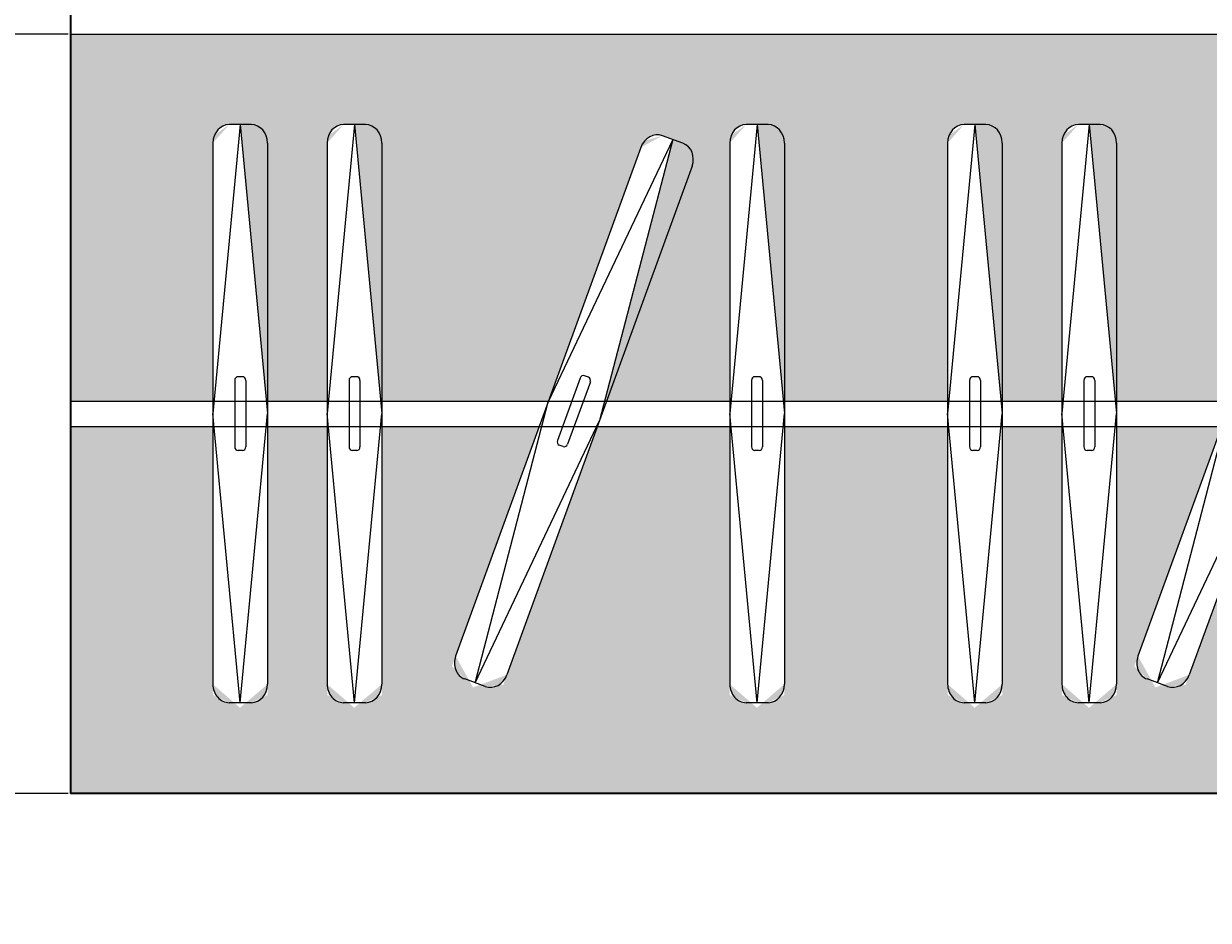
# Model space of a CAD drawing. Units: millimetres. Extents: x 27017497 to 27018854, y 7058029 to 7059154.
# Tile 38 of 91: x 27017621 to 27017655, y 7058433 to 7058459. Entities that reach past the tile are written whole.
import ezdxf

# ---------------------------------------------------------------- set-up
doc = ezdxf.new("R2010")
doc.units = ezdxf.units.MM
for name, color, linetype, lineweight in [('A-ANNO-DIMS', 2, 'Continuous', 18), ('A-FLOR-CASE', 8, 'Continuous', 20), ('A-FLOR-CASE-PATT', 44, 'Continuous', 13), ('A-WALL', 7, 'Continuous', 35)]:
    doc.layers.add(name, color=color, linetype=linetype, lineweight=lineweight)
doc.styles.get("Standard").update_dxf_attribs({"font": 'arial.ttf'})
doc.dimstyles.get("Standard").update_dxf_attribs({"dimtxt": 0.18, "dimasz": 0.18, "dimexe": 0.18, "dimexo": 0.0625, "dimgap": 0.09, "dimtad": 0, "dimtih": 1, "dimtoh": 1, "dimdec": 4, "dimzin": 0, "dimdsep": 46, "dimtxsty": 'Standard', "dimcen": 0.09, "dimadec": 0, "dimazin": 0, "dimtfac": 1, "dimtdec": 4, "dimtofl": 0, "dimtmove": 0, "dimatfit": 3, "dimfxl": 1, "dimtolj": 1, "dimtzin": 0, "dimarcsym": 0})

# ---------------------------------------------------------------- blocks, each defined once
blk = doc.blocks.new('WARDROBE-HANGING-WALL-BACKED')
for p, q in [((0, 21.737), (65.212, 21.737)), ((0, 0), (0, 21.737)), ((4.862, 19.152), (4.08, 10.877)), ((5.175, 19.152), (4.549, 19.152)), ((4.862, 19.152), (5.645, 10.877)), ((8.135, 19.152), (7.353, 10.877)), ((8.448, 19.152), (7.822, 19.152)), ((8.135, 19.152), (8.918, 10.877)), ((19.663, 19.152), (18.88, 10.877)), ((19.976, 19.152), (19.35, 19.152)), ((19.663, 19.152), (20.445, 10.877)), ((25.9, 19.152), (25.118, 10.877)), ((26.213, 19.152), (25.587, 19.152)), ((25.9, 19.152), (26.683, 10.877)), ((29.173, 19.152), (28.391, 10.877)), ((29.486, 19.152), (28.86, 19.152)), ((29.173, 19.152), (29.956, 10.877)), ((17.246, 18.725), (13.68, 11.217)), ((17.246, 18.725), (15.151, 10.682)), ((17.54, 18.618), (16.952, 18.833)), ((4.08, 18.624), (4.08, 3.13)), ((5.645, 18.624), (5.645, 3.13)), ((7.353, 18.624), (7.353, 3.13)), ((8.918, 18.624), (8.918, 3.13)), ((16.33, 18.497), (11.03, 3.937)), ((18.88, 18.624), (18.88, 3.13)), ((20.445, 18.624), (20.445, 3.13)), ((25.118, 18.624), (25.118, 3.13)), ((26.683, 18.624), (26.683, 3.13)), ((28.391, 18.624), (28.391, 3.13)), ((29.956, 18.624), (29.956, 3.13)), ((35.867, 18.497), (30.567, 3.937)), ((17.8, 17.961), (12.501, 3.402)), ((37.337, 17.961), (32.038, 3.402)), ((4.925, 11.933), (4.8, 11.933)), ((8.198, 11.933), (8.073, 11.933)), ((14.594, 11.896), (13.943, 10.109)), ((14.836, 11.92), (14.718, 11.963)), ((19.725, 11.933), (19.6, 11.933)), ((25.963, 11.933), (25.838, 11.933)), ((29.236, 11.933), (29.111, 11.933)), ((4.706, 11.828), (4.706, 9.926)), ((5.019, 11.828), (5.019, 9.926)), ((7.979, 11.828), (7.979, 9.926)), ((8.292, 11.828), (8.292, 9.926)), ((14.888, 11.789), (14.237, 10.002)), ((19.506, 11.828), (19.506, 9.926)), ((19.819, 11.828), (19.819, 9.926)), ((25.744, 11.828), (25.744, 9.926)), ((26.057, 11.828), (26.057, 9.926)), ((29.017, 11.828), (29.017, 9.926)), ((29.33, 11.828), (29.33, 9.926)), ((0, 11.231), (65.212, 11.231)), ((11.585, 3.173), (13.68, 11.217)), ((31.122, 3.173), (33.217, 11.217)), ((4.862, 2.602), (4.08, 10.877)), ((4.862, 2.602), (5.645, 10.877)), ((8.135, 2.602), (7.353, 10.877)), ((8.135, 2.602), (8.918, 10.877)), ((19.663, 2.602), (18.88, 10.877)), ((19.663, 2.602), (20.445, 10.877)), ((25.9, 2.602), (25.118, 10.877)), ((25.9, 2.602), (26.683, 10.877)), ((29.173, 2.602), (28.391, 10.877)), ((29.173, 2.602), (29.956, 10.877)), ((11.585, 3.173), (15.151, 10.682)), ((31.122, 3.173), (34.688, 10.682)), ((0, 10.506), (65.212, 10.506)), ((14.113, 9.935), (13.995, 9.978)), ((4.925, 9.821), (4.8, 9.821)), ((8.198, 9.821), (8.073, 9.821)), ((19.725, 9.821), (19.6, 9.821)), ((25.963, 9.821), (25.838, 9.821)), ((29.236, 9.821), (29.111, 9.821)), ((11.879, 3.066), (11.291, 3.28)), ((31.416, 3.066), (30.828, 3.28)), ((5.175, 2.602), (4.549, 2.602)), ((8.448, 2.602), (7.822, 2.602)), ((19.976, 2.602), (19.35, 2.602)), ((26.213, 2.602), (25.587, 2.602)), ((29.486, 2.602), (28.86, 2.602))]:
    blk.add_line(p, q)
for centre, major_axis, start_param, end_param in [((4.549, 18.624), (0, 0.528), 0, 1.570796), ((5.175, 18.624), (0, 0.528), 4.712389, 6.283185), ((7.822, 18.624), (0, 0.528), 0, 1.570796), ((8.448, 18.624), (0, 0.528), 4.712389, 6.283185), ((19.35, 18.624), (0, 0.528), 0, 1.570796), ((19.976, 18.624), (0, 0.528), 4.712389, 6.283185), ((25.587, 18.624), (0, 0.528), 0, 1.570796), ((26.213, 18.624), (0, 0.528), 4.712389, 6.283185), ((28.86, 18.624), (0, 0.528), 0, 1.570796), ((29.486, 18.624), (0, 0.528), 4.712389, 6.283185), ((16.771, 18.336), (0.181, 0.496), 0, 1.570796), ((17.359, 18.122), (0.181, 0.496), -1.570796, 0), ((4.8, 11.828), (0, 0.106), 0, 1.570796), ((4.925, 11.828), (0, 0.106), -1.570796, 0), ((8.073, 11.828), (0, 0.106), 0, 1.570796), ((8.198, 11.828), (0, 0.106), -1.570796, 0), ((14.682, 11.864), (0.0361, 0.0993), 0, 1.570796), ((14.799, 11.821), (0.0361, 0.0993), 4.712389, 6.283185), ((19.6, 11.828), (0, 0.106), 0, 1.570796), ((19.725, 11.828), (0, 0.106), -1.570796, 0), ((25.838, 11.828), (0, 0.106), 0, 1.570796), ((25.963, 11.828), (0, 0.106), -1.570796, 0), ((29.111, 11.828), (0, 0.106), 0, 1.570796), ((29.236, 11.828), (0, 0.106), -1.570796, 0), ((4.8, 9.926), (0, 0.106), 1.570796, 3.141593), ((4.925, 9.926), (0, 0.106), 3.141593, 4.712389), ((8.073, 9.926), (0, 0.106), 1.570796, 3.141593), ((8.198, 9.926), (0, 0.106), 3.141593, 4.712389), ((14.031, 10.077), (0.0361, 0.0993), 1.570796, 3.141593), ((14.149, 10.034), (0.0361, 0.0993), 3.141593, 4.712389), ((19.6, 9.926), (0, 0.106), 1.570796, 3.141593), ((19.725, 9.926), (0, 0.106), 3.141593, 4.712389), ((25.838, 9.926), (0, 0.106), 1.570796, 3.141593), ((25.963, 9.926), (0, 0.106), 3.141593, 4.712389), ((29.111, 9.926), (0, 0.106), 1.570796, 3.141593), ((29.236, 9.926), (0, 0.106), 3.141593, 4.712389), ((11.472, 3.776), (0.181, 0.496), 1.570796, 3.141593), ((31.008, 3.776), (0.181, 0.496), 1.570796, 3.141593), ((12.06, 3.562), (0.181, 0.496), 3.141593, 4.712389), ((31.597, 3.562), (0.181, 0.496), 3.141593, 4.712389), ((4.549, 3.13), (0, 0.528), 1.570796, 3.141593), ((5.175, 3.13), (0, 0.528), 3.141593, 4.712389), ((7.822, 3.13), (0, 0.528), 1.570796, 3.141593), ((8.448, 3.13), (0, 0.528), 3.141593, 4.712389), ((19.35, 3.13), (0, 0.528), 1.570796, 3.141593), ((19.976, 3.13), (0, 0.528), 3.141593, 4.712389), ((25.587, 3.13), (0, 0.528), 1.570796, 3.141593), ((26.213, 3.13), (0, 0.528), 3.141593, 4.712389), ((28.86, 3.13), (0, 0.528), 1.570796, 3.141593), ((29.486, 3.13), (0, 0.528), 3.141593, 4.712389)]:
    blk.add_ellipse(centre, major_axis=major_axis, ratio=0.888892, start_param=start_param, end_param=end_param)
blk = doc.blocks.new('*D45')
at = {"layer": 'A-ANNO-DIMS', "color": 0, "lineweight": -2, "transparency": 16777216}
for p, q in [((27017622.665, 7058458.704), (27017622.665, 7058468.604)), ((27017687.877, 7058458.704), (27017687.877, 7058468.604)), ((27017622.845, 7058468.424), (27017653.586, 7058468.424)), ((27017687.697, 7058468.424), (27017656.955, 7058468.424))]:
    blk.add_line(p, q, dxfattribs=at)
at = {"layer": 'A-ANNO-DIMS', "color": 0, "transparency": 16777216}
for points in [[(27017622.845, 7058468.454), (27017622.845, 7058468.394), (27017622.665, 7058468.424)], [(27017687.697, 7058468.454), (27017687.697, 7058468.394), (27017687.877, 7058468.424)]]:
    blk.add_solid(points, dxfattribs=at)
at = {"layer": 'Defpoints', "color": 0, "transparency": 16777216}
for p in [(27017687.877, 7058468.424), (27017622.665, 7058458.642), (27017687.877, 7058458.642)]:
    blk.add_point(p, dxfattribs=at)
at = {"layer": 'A-ANNO-DIMS', "color": 0, "transparency": 16777216, "insert": (27017655.271, 7058468.424), "char_height": 0.18, "attachment_point": 5}
blk.add_mtext('\\A1;WALL WARDROBE 65 TYP.', dxfattribs=at)
blk = doc.blocks.new('*D46')
at = {"layer": 'A-ANNO-DIMS', "color": 0, "lineweight": -2, "transparency": 16777216}
for p, q in [((27017622.603, 7058458.642), (27017612.703, 7058458.642)), ((27017612.883, 7058458.462), (27017612.883, 7058447.954)), ((27017612.883, 7058437.085), (27017612.883, 7058447.593)), ((27017622.603, 7058436.905), (27017612.703, 7058436.905))]:
    blk.add_line(p, q, dxfattribs=at)
at = {"layer": 'A-ANNO-DIMS', "color": 0, "transparency": 16777216}
for points in [[(27017612.853, 7058458.462), (27017612.913, 7058458.462), (27017612.883, 7058458.642)], [(27017612.853, 7058437.085), (27017612.913, 7058437.085), (27017612.883, 7058436.905)]]:
    blk.add_solid(points, dxfattribs=at)
at = {"layer": 'Defpoints', "color": 0, "transparency": 16777216}
for p in [(27017612.883, 7058458.642), (27017622.665, 7058458.642), (27017622.665, 7058436.905)]:
    blk.add_point(p, dxfattribs=at)
at = {"layer": 'A-ANNO-DIMS', "color": 0, "transparency": 16777216, "insert": (27017612.883, 7058447.773), "char_height": 0.18, "attachment_point": 5}
blk.add_mtext('\\A1;22 TYP.', dxfattribs=at)
blk = doc.blocks.new('*D48')
at = {"layer": 'A-ANNO-DIMS', "color": 0, "lineweight": -2, "transparency": 16777216}
for p, q in [((27018463.498, 7058622.912), (27017497.536, 7058622.912)), ((27017497.716, 7058622.732), (27017497.716, 7058357.753)), ((27017497.716, 7058092.41), (27017497.716, 7058357.389)), ((27018555.129, 7058092.23), (27017497.536, 7058092.23))]:
    blk.add_line(p, q, dxfattribs=at)
at = {"layer": 'A-ANNO-DIMS', "color": 0, "transparency": 16777216}
for points in [[(27017497.686, 7058622.732), (27017497.746, 7058622.732), (27017497.716, 7058622.912)], [(27017497.686, 7058092.41), (27017497.746, 7058092.41), (27017497.716, 7058092.23)]]:
    blk.add_solid(points, dxfattribs=at)
at = {"layer": 'Defpoints', "color": 0, "transparency": 16777216}
for p in [(27018463.561, 7058622.912), (27017497.716, 7058092.23), (27018555.192, 7058092.23)]:
    blk.add_point(p, dxfattribs=at)
at = {"layer": 'A-ANNO-DIMS', "color": 0, "transparency": 16777216, "insert": (27017497.716, 7058357.571), "char_height": 0.18, "attachment_point": 5}
blk.add_mtext('\\A1;530.7', dxfattribs=at)

msp = doc.modelspace()

# ---------------------------------------------------------------- hatches: boundary and pattern name
at = {"layer": 'A-FLOR-CASE-PATT'}
h = msp.add_hatch(color=256, dxfattribs=at)
h.dxf.hatch_style = 1
edge = h.paths.add_edge_path()
edge.add_line((27017641.545, 7058447.411), (27017637.752, 7058447.411))
edge.add_line((27017637.752, 7058447.411), (27017635.06, 7058440.016))
edge.add_ellipse((27017634.725, 7058440.467), major_axis=(0.181, 0.496), ratio=0.888892, start_angle=180, end_angle=270, ccw=False)
edge.add_line((27017634.184, 7058439.939), (27017634.19, 7058439.951))
edge.add_ellipse((27017634.137, 7058440.681), major_axis=(0.181, 0.496), ratio=0.888892, start_angle=90, end_angle=180, ccw=False)
edge.add_line((27017633.59, 7058440.551), (27017636.086, 7058447.411))
edge.add_line((27017636.086, 7058447.411), (27017631.583, 7058447.411))
edge.add_line((27017631.583, 7058447.411), (27017631.583, 7058439.726))
edge.add_ellipse((27017631.113, 7058440.035), major_axis=(0, 0.528), ratio=0.888892, start_angle=180, end_angle=270, ccw=False)
edge.add_line((27017630.786, 7058439.354), (27017630.787, 7058439.367))
edge.add_ellipse((27017630.487, 7058440.035), major_axis=(0, 0.528), ratio=0.888892, start_angle=90, end_angle=180, ccw=False)
edge.add_line((27017630.018, 7058439.726), (27017630.018, 7058447.411))
edge.add_line((27017630.018, 7058447.411), (27017628.31, 7058447.411))
edge.add_line((27017628.31, 7058447.411), (27017628.31, 7058439.726))
edge.add_ellipse((27017627.84, 7058440.035), major_axis=(0, 0.528), ratio=0.888892, start_angle=180, end_angle=270, ccw=False)
edge.add_line((27017627.513, 7058439.354), (27017627.514, 7058439.367))
edge.add_ellipse((27017627.214, 7058440.035), major_axis=(0, 0.528), ratio=0.888892, start_angle=90, end_angle=180, ccw=False)
edge.add_line((27017626.745, 7058439.726), (27017626.745, 7058447.411))
edge.add_line((27017626.745, 7058447.411), (27017622.666, 7058447.411))
edge.add_line((27017622.666, 7058447.411), (27017622.666, 7058436.912))
edge.add_line((27017622.666, 7058436.912), (27017687.877, 7058436.912))
edge.add_line((27017687.877, 7058436.912), (27017687.877, 7058447.411))
edge.add_line((27017687.877, 7058447.411), (27017685.741, 7058447.411))
edge.add_line((27017685.741, 7058447.411), (27017685.741, 7058439.726))
edge.add_ellipse((27017685.271, 7058440.035), major_axis=(0, 0.528), ratio=0.888892, start_angle=180, end_angle=270, ccw=False)
edge.add_line((27017684.944, 7058439.354), (27017684.945, 7058439.367))
edge.add_ellipse((27017684.645, 7058440.035), major_axis=(0, 0.528), ratio=0.888892, start_angle=90, end_angle=180, ccw=False)
edge.add_line((27017684.176, 7058439.726), (27017684.176, 7058447.411))
edge.add_line((27017684.176, 7058447.411), (27017680.383, 7058447.411))
edge.add_line((27017680.383, 7058447.411), (27017677.691, 7058440.016))
edge.add_ellipse((27017677.356, 7058440.467), major_axis=(0.181, 0.496), ratio=0.888892, start_angle=180, end_angle=270, ccw=False)
edge.add_line((27017676.815, 7058439.939), (27017676.821, 7058439.951))
edge.add_ellipse((27017676.767, 7058440.681), major_axis=(0.181, 0.496), ratio=0.888892, start_angle=90, end_angle=180, ccw=False)
edge.add_line((27017676.22, 7058440.551), (27017678.717, 7058447.411))
edge.add_line((27017678.717, 7058447.411), (27017674.214, 7058447.411))
edge.add_line((27017674.214, 7058447.411), (27017674.214, 7058439.726))
edge.add_ellipse((27017673.744, 7058440.035), major_axis=(0, 0.528), ratio=0.888892, start_angle=180, end_angle=270, ccw=False)
edge.add_line((27017673.417, 7058439.354), (27017673.418, 7058439.367))
edge.add_ellipse((27017673.118, 7058440.035), major_axis=(0, 0.528), ratio=0.888892, start_angle=90, end_angle=180, ccw=False)
edge.add_line((27017672.649, 7058439.726), (27017672.649, 7058447.411))
edge.add_line((27017672.649, 7058447.411), (27017670.94, 7058447.411))
edge.add_line((27017670.94, 7058447.411), (27017670.94, 7058439.726))
edge.add_ellipse((27017670.471, 7058440.035), major_axis=(0, 0.528), ratio=0.888892, start_angle=180, end_angle=270, ccw=False)
edge.add_line((27017670.143, 7058439.354), (27017670.145, 7058439.367))
edge.add_ellipse((27017669.845, 7058440.035), major_axis=(0, 0.528), ratio=0.888892, start_angle=90, end_angle=180, ccw=False)
edge.add_line((27017669.375, 7058439.726), (27017669.375, 7058447.411))
edge.add_line((27017669.375, 7058447.411), (27017663.036, 7058447.411))
edge.add_line((27017663.036, 7058447.411), (27017663.036, 7058439.726))
edge.add_ellipse((27017662.567, 7058440.035), major_axis=(0, 0.528), ratio=0.888892, start_angle=180, end_angle=270, ccw=False)
edge.add_line((27017662.239, 7058439.354), (27017662.241, 7058439.367))
edge.add_ellipse((27017661.941, 7058440.035), major_axis=(0, 0.528), ratio=0.888892, start_angle=90, end_angle=180, ccw=False)
edge.add_line((27017661.471, 7058439.726), (27017661.471, 7058447.411))
edge.add_line((27017661.471, 7058447.411), (27017657.289, 7058447.411))
edge.add_line((27017657.289, 7058447.411), (27017654.597, 7058440.016))
edge.add_ellipse((27017654.262, 7058440.467), major_axis=(0.181, 0.496), ratio=0.888892, start_angle=180, end_angle=270, ccw=False)
edge.add_line((27017653.721, 7058439.939), (27017653.727, 7058439.951))
edge.add_ellipse((27017653.673, 7058440.681), major_axis=(0.181, 0.496), ratio=0.888892, start_angle=90, end_angle=180, ccw=False)
edge.add_line((27017653.126, 7058440.551), (27017655.623, 7058447.411))
edge.add_line((27017655.623, 7058447.411), (27017652.621, 7058447.411))
edge.add_line((27017652.621, 7058447.411), (27017652.621, 7058439.726))
edge.add_ellipse((27017652.151, 7058440.035), major_axis=(0, 0.528), ratio=0.888892, start_angle=180, end_angle=270, ccw=False)
edge.add_line((27017651.824, 7058439.354), (27017651.825, 7058439.367))
edge.add_ellipse((27017651.525, 7058440.035), major_axis=(0, 0.528), ratio=0.888892, start_angle=90, end_angle=180, ccw=False)
edge.add_line((27017651.056, 7058439.726), (27017651.056, 7058447.411))
edge.add_line((27017651.056, 7058447.411), (27017649.348, 7058447.411))
edge.add_line((27017649.348, 7058447.411), (27017649.348, 7058439.726))
edge.add_ellipse((27017648.878, 7058440.035), major_axis=(0, 0.528), ratio=0.888892, start_angle=180, end_angle=270, ccw=False)
edge.add_line((27017648.551, 7058439.354), (27017648.552, 7058439.367))
edge.add_ellipse((27017648.252, 7058440.035), major_axis=(0, 0.528), ratio=0.888892, start_angle=90, end_angle=180, ccw=False)
edge.add_line((27017647.783, 7058439.726), (27017647.783, 7058447.411))
edge.add_line((27017647.783, 7058447.411), (27017643.11, 7058447.411))
edge.add_line((27017643.11, 7058447.411), (27017643.11, 7058439.726))
edge.add_ellipse((27017642.641, 7058440.035), major_axis=(0, 0.528), ratio=0.888892, start_angle=180, end_angle=270, ccw=False)
edge.add_line((27017642.313, 7058439.354), (27017642.314, 7058439.367))
edge.add_ellipse((27017642.015, 7058440.035), major_axis=(0, 0.528), ratio=0.888892, start_angle=90, end_angle=180, ccw=False)
edge.add_line((27017641.545, 7058439.726), (27017641.545, 7058447.411))
edge = h.paths.add_edge_path()
edge.add_line((27017669.845, 7058456.057), (27017670.158, 7058456.057))
edge.add_line((27017670.158, 7058456.057), (27017670.907, 7058448.136))
edge.add_line((27017670.907, 7058448.136), (27017672.649, 7058448.136))
edge.add_line((27017672.649, 7058448.136), (27017672.649, 7058455.723))
edge.add_ellipse((27017673.118, 7058455.529), major_axis=(0, 0.528), ratio=0.888892, start_angle=0, end_angle=90, ccw=False)
edge.add_line((27017673.118, 7058456.057), (27017673.431, 7058456.057))
edge.add_line((27017673.431, 7058456.057), (27017674.18, 7058448.136))
edge.add_line((27017674.18, 7058448.136), (27017678.981, 7058448.136))
edge.add_line((27017678.981, 7058448.136), (27017681.692, 7058455.583))
edge.add_ellipse((27017682.067, 7058455.241), major_axis=(0.181, 0.496), ratio=0.888892, start_angle=0, end_angle=90, ccw=False)
edge.add_line((27017682.247, 7058455.738), (27017682.542, 7058455.63))
edge.add_line((27017682.542, 7058455.63), (27017680.59, 7058448.136))
edge.add_line((27017680.59, 7058448.136), (27017684.176, 7058448.136))
edge.add_line((27017684.176, 7058448.136), (27017684.176, 7058455.723))
edge.add_ellipse((27017684.645, 7058455.529), major_axis=(0, 0.528), ratio=0.888892, start_angle=0, end_angle=90, ccw=False)
edge.add_line((27017684.645, 7058456.057), (27017684.958, 7058456.057))
edge.add_line((27017684.958, 7058456.057), (27017685.707, 7058448.136))
edge.add_line((27017685.707, 7058448.136), (27017687.877, 7058448.136))
edge.add_line((27017687.877, 7058448.136), (27017687.877, 7058458.642))
edge.add_line((27017687.877, 7058458.642), (27017622.666, 7058458.642))
edge.add_line((27017622.666, 7058458.642), (27017622.666, 7058448.136))
edge.add_line((27017622.666, 7058448.136), (27017626.745, 7058448.136))
edge.add_line((27017626.745, 7058448.136), (27017626.745, 7058455.723))
edge.add_ellipse((27017627.214, 7058455.529), major_axis=(0, 0.528), ratio=0.888892, start_angle=0, end_angle=90, ccw=False)
edge.add_line((27017627.214, 7058456.057), (27017627.527, 7058456.057))
edge.add_line((27017627.527, 7058456.057), (27017628.276, 7058448.136))
edge.add_line((27017628.276, 7058448.136), (27017630.018, 7058448.136))
edge.add_line((27017630.018, 7058448.136), (27017630.018, 7058455.723))
edge.add_ellipse((27017630.487, 7058455.529), major_axis=(0, 0.528), ratio=0.888892, start_angle=0, end_angle=90, ccw=False)
edge.add_line((27017630.487, 7058456.057), (27017630.8, 7058456.057))
edge.add_line((27017630.8, 7058456.057), (27017631.549, 7058448.136))
edge.add_line((27017631.549, 7058448.136), (27017636.35, 7058448.136))
edge.add_line((27017636.35, 7058448.136), (27017639.061, 7058455.583))
edge.add_ellipse((27017639.436, 7058455.241), major_axis=(0.181, 0.496), ratio=0.888892, start_angle=0, end_angle=90, ccw=False)
edge.add_line((27017639.617, 7058455.738), (27017639.911, 7058455.63))
edge.add_line((27017639.911, 7058455.63), (27017637.959, 7058448.136))
edge.add_line((27017637.959, 7058448.136), (27017641.545, 7058448.136))
edge.add_line((27017641.545, 7058448.136), (27017641.545, 7058455.723))
edge.add_ellipse((27017642.015, 7058455.529), major_axis=(0, 0.528), ratio=0.888892, start_angle=0, end_angle=90, ccw=False)
edge.add_line((27017642.015, 7058456.057), (27017642.328, 7058456.057))
edge.add_line((27017642.328, 7058456.057), (27017643.077, 7058448.136))
edge.add_line((27017643.077, 7058448.136), (27017647.783, 7058448.136))
edge.add_line((27017647.783, 7058448.136), (27017647.783, 7058455.723))
edge.add_ellipse((27017648.252, 7058455.529), major_axis=(0, 0.528), ratio=0.888892, start_angle=0, end_angle=90, ccw=False)
edge.add_line((27017648.252, 7058456.057), (27017648.565, 7058456.057))
edge.add_line((27017648.565, 7058456.057), (27017649.314, 7058448.136))
edge.add_line((27017649.314, 7058448.136), (27017651.056, 7058448.136))
edge.add_line((27017651.056, 7058448.136), (27017651.056, 7058455.723))
edge.add_ellipse((27017651.525, 7058455.529), major_axis=(0, 0.528), ratio=0.888892, start_angle=0, end_angle=90, ccw=False)
edge.add_line((27017651.525, 7058456.057), (27017651.838, 7058456.057))
edge.add_line((27017651.838, 7058456.057), (27017652.587, 7058448.136))
edge.add_line((27017652.587, 7058448.136), (27017655.887, 7058448.136))
edge.add_line((27017655.887, 7058448.136), (27017658.598, 7058455.583))
edge.add_ellipse((27017658.973, 7058455.241), major_axis=(0.181, 0.496), ratio=0.888892, start_angle=0, end_angle=90, ccw=False)
edge.add_line((27017659.153, 7058455.738), (27017659.448, 7058455.63))
edge.add_line((27017659.448, 7058455.63), (27017657.496, 7058448.136))
edge.add_line((27017657.496, 7058448.136), (27017661.471, 7058448.136))
edge.add_line((27017661.471, 7058448.136), (27017661.471, 7058455.723))
edge.add_ellipse((27017661.941, 7058455.529), major_axis=(0, 0.528), ratio=0.888892, start_angle=0, end_angle=90, ccw=False)
edge.add_line((27017661.941, 7058456.057), (27017662.254, 7058456.057))
edge.add_line((27017662.254, 7058456.057), (27017663.003, 7058448.136))
edge.add_line((27017663.003, 7058448.136), (27017669.375, 7058448.136))
edge.add_line((27017669.375, 7058448.136), (27017669.375, 7058455.723))
edge.add_ellipse((27017669.845, 7058455.529), major_axis=(0, 0.528), ratio=0.888892, start_angle=0, end_angle=90, ccw=False)

# ---------------------------------------------------------------- linework, layer by layer
at = {"layer": 'A-WALL'}
for p, q in [((27017622.666, 7058580.912), (27017622.666, 7058436.912)), ((27017622.666, 7058436.912), (27017716.811, 7058436.912))]:
    msp.add_line(p, q, dxfattribs=at)

# ---------------------------------------------------------------- block references
at = {"layer": 'A-FLOR-CASE'}
msp.add_blockref('WARDROBE-HANGING-WALL-BACKED', (27017622.665, 7058436.905), dxfattribs=at)

# ---------------------------------------------------------------- dimensions: what is measured, and where the dimension line sits
at = {"layer": 'A-ANNO-DIMS'}
dim = msp.add_linear_dim(base=(27017497.716, 7058092.23), p1=(27018463.561, 7058622.912), p2=(27018555.192, 7058092.23), angle=90, dimstyle='Standard', override={"dimdec": 1, "dimlfac": 1, "dimrnd": 0, "dimzin": 0, "dimdsep": 46, "dimlunit": 2}, dxfattribs=at)
dim.commit()
dim.dimension.update_dxf_attribs({"geometry": '*D48', "text_midpoint": (27017497.716, 7058357.571)})
dim = msp.add_linear_dim(base=(27017687.877, 7058468.424), p1=(27017622.665, 7058458.642), p2=(27017687.877, 7058458.642), text='WALL WARDROBE <> TYP.', dimstyle='Standard', override={"dimdec": 0, "dimlfac": 1, "dimrnd": 0, "dimzin": 0, "dimdsep": 46, "dimlunit": 2}, dxfattribs=at)
dim.commit()
dim.dimension.update_dxf_attribs({"geometry": '*D45', "text_midpoint": (27017655.271, 7058468.424)})
dim = msp.add_linear_dim(base=(27017612.883, 7058458.642), p1=(27017622.665, 7058436.905), p2=(27017622.665, 7058458.642), angle=90, text='<> TYP.', dimstyle='Standard', override={"dimdec": 0, "dimlfac": 1, "dimrnd": 0, "dimzin": 0, "dimdsep": 46, "dimlunit": 2}, dxfattribs=at)
dim.commit()
dim.dimension.update_dxf_attribs({"geometry": '*D46', "text_midpoint": (27017612.883, 7058447.773)})

doc.saveas('drawing.dxf')
